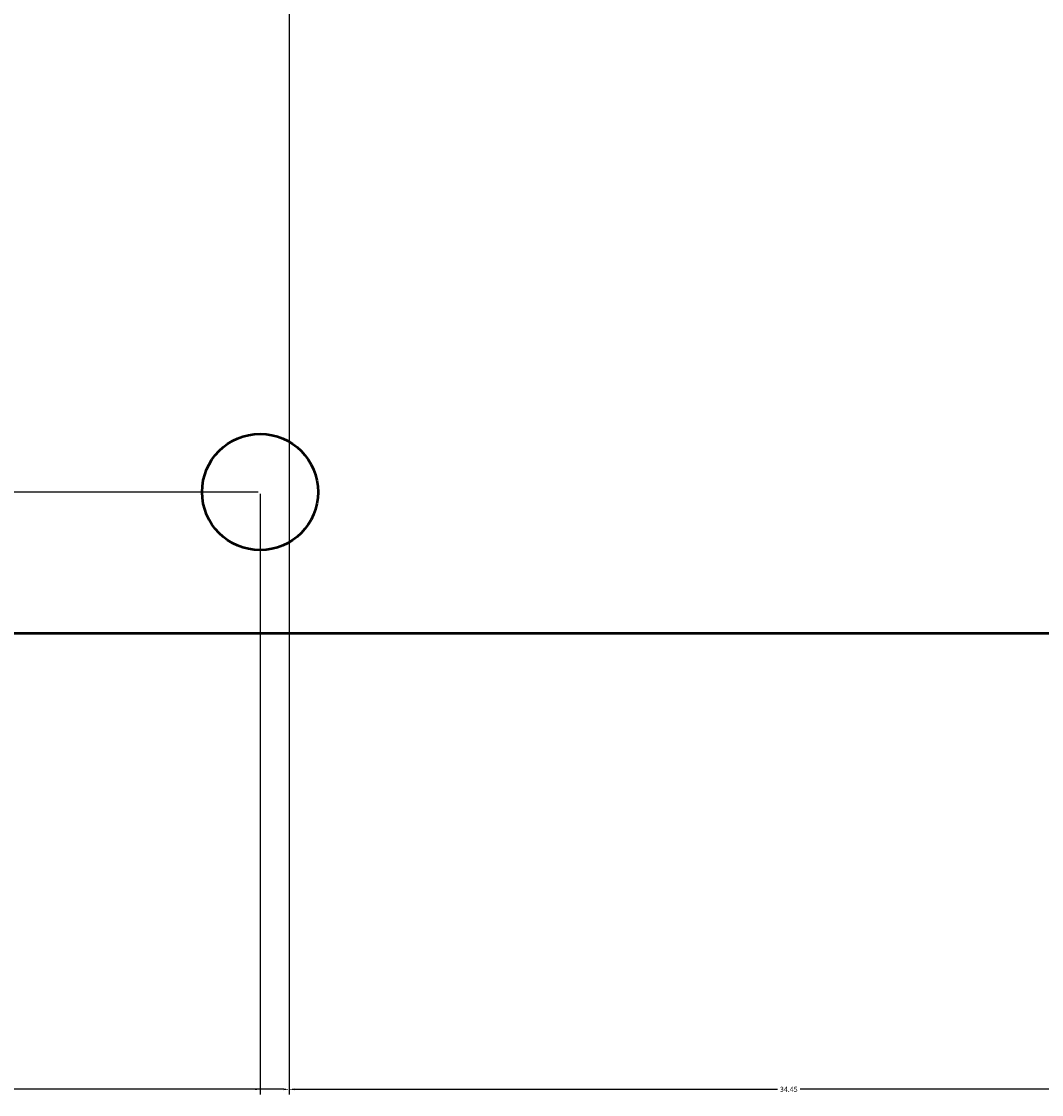
# Model space of a CAD drawing. Units: inches. Extents: x -14 to 108, y -9 to 83.
# Tile 7 of 13: x 38 to 73, y -9 to 28. Entities that reach past the tile are written whole.
import ezdxf

# ---------------------------------------------------------------- set-up
doc = ezdxf.new("R2010")
doc.units = ezdxf.units.IN
doc.header["$MEASUREMENT"] = 0
doc.layers.add('M-DIMS', color=2, linetype='Continuous', lineweight=18)
doc.layers.add('M-OUTL', color=7, linetype='Continuous', lineweight=50)
doc.styles.get("Standard").update_dxf_attribs({"font": 'arial.ttf'})
doc.dimstyles.get("Standard").update_dxf_attribs({"dimtxt": 0.18, "dimasz": 0.18, "dimexe": 0.18, "dimexo": 0.0625, "dimgap": 0.09, "dimtad": 0, "dimtih": 1, "dimtoh": 1, "dimzin": 0, "dimdsep": 46, "dimtxsty": 'Standard', "dimcen": 0.09, "dimadec": 0, "dimazin": 0, "dimtfac": 1, "dimtofl": 0, "dimtmove": 0, "dimatfit": 3, "dimfxl": 1, "dimtolj": 1, "dimtzin": 0, "dimarcsym": 0})

# ---------------------------------------------------------------- blocks, each defined once
blk = doc.blocks.new('HOLE-D4')
blk.add_circle((2, 2), 2)
blk = doc.blocks.new('*D7')
at = {"layer": 'Defpoints', "color": 0, "transparency": 16777216}
for p in [(47.098, 37.119), (5.951, 18.227), (47.098, -8.596)]:
    blk.add_point(p, dxfattribs=at)
at = {"layer": 'M-DIMS', "color": 0, "lineweight": -2, "transparency": 16777216}
for p, q in [((47.098, 37.057), (47.098, -8.776)), ((5.951, 18.165), (5.951, -8.776)), ((6.131, -8.596), (26.126, -8.596)), ((46.918, -8.596), (26.922, -8.596))]:
    blk.add_line(p, q, dxfattribs=at)
at = {"layer": 'M-DIMS', "color": 0, "transparency": 16777216}
for points in [[(6.131, -8.566), (6.131, -8.626), (5.951, -8.596)], [(46.918, -8.566), (46.918, -8.626), (47.098, -8.596)]]:
    blk.add_solid(points, dxfattribs=at)
at = {"layer": 'M-DIMS', "color": 0, "transparency": 16777216, "insert": (26.524, -8.596), "char_height": 0.18, "attachment_point": 5}
blk.add_mtext('\\A1;41.15', dxfattribs=at)
blk = doc.blocks.new('*D8')
at = {"layer": 'Defpoints', "color": 0, "transparency": 16777216}
for p in [(47.098, 37.119), (81.545, 18.227), (81.545, -8.596)]:
    blk.add_point(p, dxfattribs=at)
at = {"layer": 'M-DIMS', "color": 0, "lineweight": -2, "transparency": 16777216}
for p, q in [((47.098, 37.057), (47.098, -8.776)), ((81.545, 18.165), (81.545, -8.776)), ((47.278, -8.596), (63.927, -8.596)), ((81.365, -8.596), (64.716, -8.596))]:
    blk.add_line(p, q, dxfattribs=at)
at = {"layer": 'M-DIMS', "color": 0, "transparency": 16777216}
for points in [[(47.278, -8.566), (47.278, -8.626), (47.098, -8.596)], [(81.365, -8.566), (81.365, -8.626), (81.545, -8.596)]]:
    blk.add_solid(points, dxfattribs=at)
at = {"layer": 'M-DIMS', "color": 0, "transparency": 16777216, "insert": (64.321, -8.596), "char_height": 0.18, "attachment_point": 5}
blk.add_mtext('\\A1;34.45', dxfattribs=at)
blk = doc.blocks.new('*D11')
at = {"layer": 'Defpoints', "color": 0, "transparency": 16777216}
for p in [(47.098, 37.119), (107.813, 37.119), (86.478, 18.227)]:
    blk.add_point(p, dxfattribs=at)
at = {"layer": 'M-DIMS', "color": 0, "lineweight": -2, "transparency": 16777216}
for p, q in [((47.16, 37.119), (107.993, 37.119)), ((107.813, 36.939), (107.813, 27.855)), ((107.813, 18.407), (107.813, 27.491)), ((86.541, 18.227), (107.993, 18.227))]:
    blk.add_line(p, q, dxfattribs=at)
at = {"layer": 'M-DIMS', "color": 0, "transparency": 16777216}
for points in [[(107.783, 36.939), (107.843, 36.939), (107.813, 37.119)], [(107.783, 18.407), (107.843, 18.407), (107.813, 18.227)]]:
    blk.add_solid(points, dxfattribs=at)
at = {"layer": 'M-DIMS', "color": 0, "transparency": 16777216, "insert": (107.813, 27.673), "char_height": 0.18, "attachment_point": 5}
blk.add_mtext('\\A1;18.892', dxfattribs=at)
blk = doc.blocks.new('*D17')
at = {"layer": 'Defpoints', "color": 0, "transparency": 16777216}
for p in [(27.381, 15.402), (46.1, 11.987), (46.1, -8.596)]:
    blk.add_point(p, dxfattribs=at)
at = {"layer": 'M-DIMS', "color": 0, "lineweight": -2, "transparency": 16777216}
for p, q in [((27.381, 15.34), (27.381, -8.776)), ((46.1, 11.925), (46.1, -8.776)), ((27.561, -8.596), (36.356, -8.596)), ((45.92, -8.596), (37.125, -8.596))]:
    blk.add_line(p, q, dxfattribs=at)
at = {"layer": 'M-DIMS', "color": 0, "transparency": 16777216}
for points in [[(27.561, -8.566), (27.561, -8.626), (27.381, -8.596)], [(45.92, -8.566), (45.92, -8.626), (46.1, -8.596)]]:
    blk.add_solid(points, dxfattribs=at)
at = {"layer": 'M-DIMS', "color": 0, "transparency": 16777216, "insert": (36.741, -8.596), "char_height": 0.18, "attachment_point": 5}
blk.add_mtext('\\A1;18.72', dxfattribs=at)
blk = doc.blocks.new('*D20')
at = {"layer": 'Defpoints', "color": 0, "transparency": 16777216}
for p in [(-13.617, 15.402), (27.381, 15.402), (46.1, 11.987)]:
    blk.add_point(p, dxfattribs=at)
at = {"layer": 'M-DIMS', "color": 0, "lineweight": -2, "transparency": 16777216}
for p, q in [((27.318, 15.402), (-13.797, 15.402)), ((-13.617, 15.222), (-13.617, 13.877)), ((-13.617, 12.167), (-13.617, 13.513)), ((46.038, 11.987), (-13.797, 11.987))]:
    blk.add_line(p, q, dxfattribs=at)
at = {"layer": 'M-DIMS', "color": 0, "transparency": 16777216}
for points in [[(-13.647, 15.222), (-13.587, 15.222), (-13.617, 15.402)], [(-13.647, 12.167), (-13.587, 12.167), (-13.617, 11.987)]]:
    blk.add_solid(points, dxfattribs=at)
at = {"layer": 'M-DIMS', "color": 0, "transparency": 16777216, "insert": (-13.617, 13.695), "char_height": 0.18, "attachment_point": 5}
blk.add_mtext('\\A1;3.415', dxfattribs=at)

msp = doc.modelspace()

# ---------------------------------------------------------------- linework, layer by layer
at = {"layer": 'M-OUTL'}
msp.add_lwpolyline([(12.0979, 7.1193), (82.0979, 7.1193)], dxfattribs=at)

# ---------------------------------------------------------------- block references
msp.add_blockref('HOLE-D4', (44.1005, 9.9867), dxfattribs=at)

# ---------------------------------------------------------------- dimensions: what is measured, and where the dimension line sits
at = {"layer": 'M-DIMS'}
for base, p1, p2, picture, middle in [((47.0979, -8.5957), (5.9508, 18.2274), (47.0979, 37.1193), '*D7', (26.5244, -8.5957)), ((81.5446, -8.5957), (47.0979, 37.1193), (81.5446, 18.2274), '*D8', (64.3213, -8.5957)), ((46.1003, -8.5957), (27.3809, 15.4023), (46.1003, 11.987), '*D17', (36.7406, -8.5957))]:
    dim = msp.add_linear_dim(base=base, p1=p1, p2=p2, dimstyle='Standard', override={"dimdec": 2, "dimlfac": 1, "dimrnd": 0, "dimzin": 0, "dimdsep": 46, "dimlunit": 2}, dxfattribs=at)
    dim.commit()
    dim.dimension.update_dxf_attribs({"geometry": picture, "text_midpoint": middle})
for base, p1, p2, picture, middle in [((107.8129, 37.1193), (86.4784, 18.2274), (47.0979, 37.1193), '*D11', (107.8129, 27.6733)), ((-13.6171, 15.4023), (46.1003, 11.987), (27.3809, 15.4023), '*D20', (-13.6171, 13.6947))]:
    dim = msp.add_linear_dim(base=base, p1=p1, p2=p2, angle=90, dimstyle='Standard', override={"dimdec": 3, "dimlfac": 1, "dimrnd": 0, "dimzin": 0, "dimdsep": 46, "dimlunit": 2}, dxfattribs=at)
    dim.commit()
    dim.dimension.update_dxf_attribs({"geometry": picture, "text_midpoint": middle})

doc.saveas('drawing.dxf')
